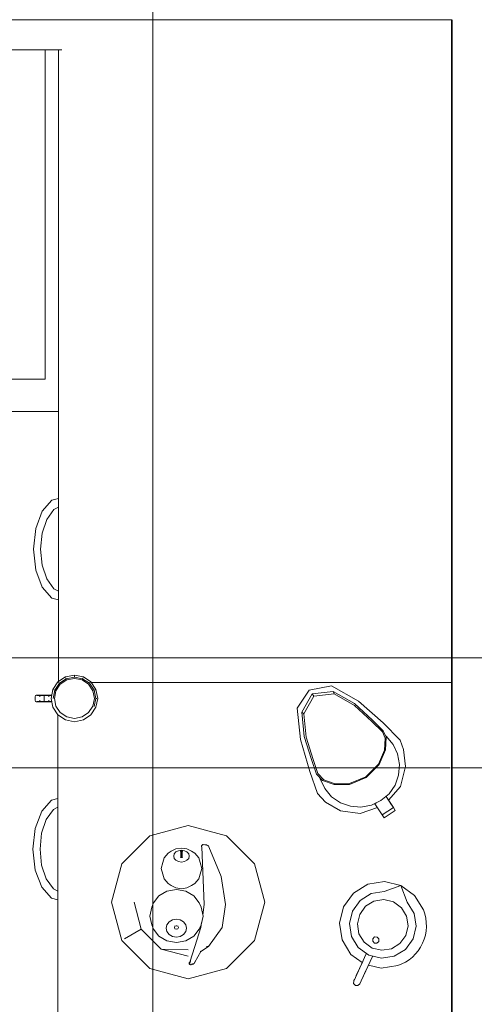
# Model space of a CAD drawing. Units: feet. Extents: x -297 to 770, y -228 to 625.
# Tile 12 of 14: x 716 to 734, y 194 to 233. Entities that reach past the tile are written whole.
import ezdxf

# ---------------------------------------------------------------- set-up
doc = ezdxf.new("R2010")
doc.units = ezdxf.units.FT
doc.header["$MEASUREMENT"] = 0
for name, color, linetype, lineweight in [('A-ANNO-DIMS', 2, 'Continuous', 18), ('A-EQPM', 8, 'Continuous', 13), ('A-FLOR-CASE', 8, 'Continuous', 18), ('A-FLOR-FIXT', 8, 'Continuous', 18), ('A-WALL', 7, 'Continuous', 35), ('windows', 30, 'Continuous', 18)]:
    doc.layers.add(name, color=color, linetype=linetype, lineweight=lineweight)
doc.styles.get("Standard").update_dxf_attribs({"font": 'arial.ttf'})
doc.dimstyles.get("Standard").update_dxf_attribs({"dimtxt": 3, "dimasz": 2, "dimexe": 0.18, "dimexo": 0.0625, "dimgap": 0.09, "dimtad": 1, "dimtoh": 1, "dimdec": 1, "dimzin": 0, "dimdsep": 46, "dimlunit": 3, "dimtxsty": 'Standard', "dimcen": 0, "dimclre": 256, "dimadec": 0, "dimazin": 0, "dimtfac": 1, "dimtdec": 1, "dimtofl": 0, "dimtmove": 0, "dimatfit": 3, "dimfxl": 1, "dimtolj": 1, "dimtzin": 0, "dimlwe": -1, "dimarcsym": 0})

# ---------------------------------------------------------------- blocks, each defined once
blk = doc.blocks.new('WIN-5FT')
blk.add_lwpolyline([(60, 0), (60, 9), (0, 9), (0, 0)], close=True)
blk = doc.blocks.new('*D54')
at = {"layer": 'A-ANNO-DIMS', "transparency": 16777216}
for p, q in [((733.096, 233.463), (354.525, 233.463)), ((733.093, 203.463), (354.525, 203.463))]:
    blk.add_line(p, q, dxfattribs=at)
at = {"layer": 'A-ANNO-DIMS', "color": 0, "lineweight": -2, "transparency": 16777216}
blk.add_line((354.705, 205.463), (354.705, 231.463), dxfattribs=at)
at = {"layer": 'A-ANNO-DIMS', "color": 0, "transparency": 16777216}
for points in [[(354.372, 231.463), (355.039, 231.463), (354.705, 233.463)], [(354.372, 205.463), (355.039, 205.463), (354.705, 203.463)]]:
    blk.add_solid(points, dxfattribs=at)
at = {"layer": 'Defpoints', "color": 0, "transparency": 16777216}
for p in [(354.705, 233.463), (733.158, 233.463), (733.155, 203.463)]:
    blk.add_point(p, dxfattribs=at)
at = {"layer": 'A-ANNO-DIMS', "color": 0, "transparency": 16777216, "insert": (353.083, 218.463), "char_height": 3, "attachment_point": 5, "rotation": 90}
blk.add_mtext('\\A1;30', dxfattribs=at)
blk = doc.blocks.new('*D68')
at = {"layer": 'A-ANNO-DIMS', "transparency": 16777216}
for p, q in [((685.155, 306.9), (685.155, -227.667)), ((721.155, 306.9), (721.155, -227.667))]:
    blk.add_line(p, q, dxfattribs=at)
at = {"layer": 'A-ANNO-DIMS', "color": 0, "lineweight": -2, "transparency": 16777216}
blk.add_line((687.155, -227.487), (719.155, -227.487), dxfattribs=at)
at = {"layer": 'A-ANNO-DIMS', "color": 0, "transparency": 16777216}
for points in [[(687.155, -227.154), (687.155, -227.821), (685.155, -227.487)], [(719.155, -227.154), (719.155, -227.821), (721.155, -227.487)]]:
    blk.add_solid(points, dxfattribs=at)
at = {"layer": 'Defpoints', "color": 0, "transparency": 16777216}
for p in [(685.155, 306.963), (721.155, 306.963), (721.155, -227.487)]:
    blk.add_point(p, dxfattribs=at)
at = {"layer": 'A-ANNO-DIMS', "color": 0, "transparency": 16777216, "insert": (703.155, -225.865), "char_height": 3, "attachment_point": 5}
blk.add_mtext('\\A1;36', dxfattribs=at)
blk = doc.blocks.new('*D75')
at = {"layer": 'A-ANNO-DIMS', "transparency": 16777216}
for p, q in [((471.753, 264.961), (769.785, 264.961)), ((471.753, 207.869), (769.785, 207.869))]:
    blk.add_line(p, q, dxfattribs=at)
at = {"layer": 'A-ANNO-DIMS', "color": 0, "lineweight": -2, "transparency": 16777216}
blk.add_line((769.605, 209.869), (769.605, 262.961), dxfattribs=at)
at = {"layer": 'A-ANNO-DIMS', "color": 0, "transparency": 16777216}
for points in [[(769.272, 262.961), (769.939, 262.961), (769.605, 264.961)], [(769.272, 209.869), (769.939, 209.869), (769.605, 207.869)]]:
    blk.add_solid(points, dxfattribs=at)
at = {"layer": 'Defpoints', "color": 0, "transparency": 16777216}
for p in [(471.691, 264.961), (769.605, 264.961), (471.691, 207.869)]:
    blk.add_point(p, dxfattribs=at)
at = {"layer": 'A-ANNO-DIMS', "color": 0, "transparency": 16777216, "insert": (767.984, 236.415), "char_height": 3, "attachment_point": 5, "rotation": 90}
blk.add_mtext('\\A1;57.09', dxfattribs=at)

msp = doc.modelspace()

# ---------------------------------------------------------------- linework, layer by layer
at = {"layer": 'A-EQPM'}
for p, q in [((726.947, 205.85), (727.438, 206.573)), ((727.438, 206.573), (728.324, 206.741)), ((728.324, 206.741), (729.408, 206.128)), ((727.141, 205.692), (727.547, 206.419)), ((727.614, 206.325), (727.222, 205.624)), ((727.547, 206.419), (728.394, 206.518)), ((727.547, 206.419), (727.614, 206.325)), ((728.43, 206.421), (727.614, 206.325)), ((728.394, 206.518), (729.252, 206.034)), ((728.394, 206.518), (728.43, 206.421)), ((729.257, 205.954), (728.43, 206.421)), ((727.084, 204.589), (726.947, 205.85)), ((729.252, 206.034), (729.972, 205.372)), ((729.951, 205.315), (729.257, 205.954)), ((730.4, 205.266), (729.408, 206.128)), ((727.235, 204.717), (727.141, 205.692)), ((727.141, 205.692), (727.222, 205.624)), ((727.222, 205.624), (727.313, 204.684)), ((729.972, 205.372), (730.407, 204.939)), ((730.371, 204.898), (729.951, 205.315)), ((731.087, 204.567), (730.4, 205.266)), ((727.084, 204.589), (727.462, 203.311)), ((727.53, 203.789), (727.235, 204.717)), ((727.313, 204.684), (727.597, 203.789)), ((730.484, 204.651), (730.371, 204.898)), ((730.407, 204.939), (730.525, 204.683)), ((730.451, 204.168), (730.484, 204.651)), ((730.525, 204.683), (730.49, 204.181)), ((730.522, 204.722), (730.5, 204.737)), ((730.798, 204.397), (730.522, 204.722)), ((731.087, 204.567), (731.221, 204.198)), ((730.211, 203.598), (730.451, 204.168)), ((730.49, 204.181), (730.241, 203.59)), ((730.981, 204.013), (730.798, 204.397)), ((731.221, 204.198), (731.296, 203.514)), ((727.725, 203.203), (727.53, 203.789)), ((727.597, 203.789), (727.785, 203.225)), ((731.058, 203.593), (730.981, 204.013)), ((729.705, 203.091), (730.211, 203.598)), ((730.241, 203.59), (729.717, 203.065)), ((731.023, 203.169), (731.058, 203.593)), ((731.296, 203.514), (731.101, 202.703)), ((727.462, 203.311), (727.772, 202.422)), ((727.97, 202.951), (727.725, 203.203)), ((727.785, 203.225), (728.021, 202.982)), ((727.866, 203.058), (727.875, 203.009)), ((727.875, 203.009), (728.058, 202.624)), ((728.021, 202.982), (728.471, 202.821)), ((729.717, 203.065), (729.045, 202.791)), ((729.058, 202.828), (729.705, 203.091)), ((730.881, 202.767), (731.023, 203.169)), ((728.437, 202.784), (727.97, 202.951)), ((728.058, 202.624), (728.334, 202.299)), ((729.045, 202.791), (728.437, 202.784)), ((728.471, 202.821), (729.058, 202.828)), ((731.101, 202.703), (730.616, 202.166)), ((730.639, 202.417), (730.881, 202.767)), ((727.772, 202.422), (728.092, 202.074)), ((728.334, 202.299), (728.685, 202.058)), ((730.314, 202.14), (730.639, 202.417)), ((730.524, 202.309), (730.476, 202.278)), ((730.742, 201.972), (730.524, 202.309)), ((730.524, 202.309), (730.603, 202.186)), ((730.814, 201.86), (730.524, 202.309)), ((728.092, 202.074), (728.686, 201.733)), ((728.685, 202.058), (729.086, 201.915)), ((729.086, 201.915), (729.511, 201.881)), ((729.486, 201.62), (730.174, 201.865)), ((729.511, 201.881), (729.93, 201.958)), ((729.93, 201.958), (730.314, 202.14)), ((730.075, 202.018), (730.123, 202.049)), ((730.365, 201.569), (730.075, 202.018)), ((730.365, 201.569), (730.814, 201.86)), ((730.814, 201.86), (730.742, 201.972)), ((730.788, 201.901), (730.814, 201.86)), ((730.814, 201.86), (730.887, 201.748)), ((728.686, 201.733), (729.486, 201.62)), ((730.438, 201.457), (730.365, 201.569)), ((730.887, 201.748), (730.438, 201.457)), ((722.574, 201.143), (721.036, 200.731)), ((722.574, 201.142), (721.037, 200.73)), ((724.111, 200.731), (722.574, 201.143)), ((724.111, 200.73), (722.574, 201.142)), ((721.036, 200.731), (719.911, 199.606)), ((721.037, 200.73), (719.912, 199.605)), ((725.237, 199.606), (724.111, 200.731)), ((725.236, 199.605), (724.111, 200.73)), ((722.308, 200.236), (722.087, 200.203)), ((722.529, 200.203), (722.308, 200.236)), ((723.111, 200.334), (723.12, 200.342)), ((723.114, 200.286), (723.111, 200.334)), ((723.111, 200.334), (723.113, 200.286)), ((723.113, 200.286), (723.114, 200.286)), ((723.114, 200.286), (723.114, 200.286)), ((723.119, 200.348), (723.134, 200.362)), ((723.146, 200.357), (723.119, 200.348)), ((723.119, 200.342), (723.119, 200.348)), ((723.224, 197.969), (723.122, 200.286)), ((723.134, 200.362), (723.139, 200.364)), ((723.134, 200.362), (723.151, 200.362)), ((723.142, 200.367), (723.139, 200.364)), ((723.139, 200.364), (723.142, 200.367)), ((723.153, 200.371), (723.142, 200.367)), ((723.171, 200.376), (723.153, 200.371)), ((723.155, 200.371), (723.171, 200.376)), ((723.16, 200.371), (723.171, 200.376)), ((723.171, 200.376), (723.168, 200.371)), ((723.171, 200.376), (723.259, 200.371)), ((723.206, 200.371), (723.171, 200.376)), ((723.171, 200.376), (723.22, 200.371)), ((723.171, 200.376), (723.179, 200.371)), ((723.259, 200.371), (723.292, 200.364)), ((723.286, 200.362), (723.27, 200.364)), ((723.312, 200.362), (723.292, 200.364)), ((723.325, 200.357), (723.312, 200.362)), ((723.344, 200.353), (723.325, 200.357)), ((723.344, 200.353), (723.372, 200.338)), ((723.383, 200.334), (723.37, 200.339)), ((723.38, 200.332), (723.383, 200.334)), ((723.383, 200.334), (723.384, 200.332)), ((723.384, 200.332), (723.39, 200.329)), ((723.39, 200.329), (723.408, 200.286)), ((723.408, 200.286), (723.395, 200.286)), ((723.898, 199.095), (723.403, 200.286)), ((721.611, 199.844), (721.554, 199.657)), ((721.775, 200.029), (721.611, 199.844)), ((721.9, 200.108), (721.775, 200.029)), ((722.087, 200.203), (721.9, 200.108)), ((722.019, 200.006), (721.996, 199.916)), ((721.996, 199.916), (722.019, 199.826)), ((722.087, 200.083), (722.019, 200.006)), ((722.019, 199.826), (722.087, 199.749)), ((722.188, 200.134), (722.087, 200.083)), ((722.308, 200.152), (722.188, 200.134)), ((722.267, 200.117), (722.279, 200.125)), ((722.279, 200.108), (722.267, 200.117)), ((722.267, 200.117), (722.279, 200.059)), ((722.279, 199.906), (722.269, 199.87)), ((722.279, 200.125), (722.308, 200.129)), ((722.287, 200.051), (722.279, 200.108)), ((722.279, 200.108), (722.308, 200.105)), ((722.279, 200.059), (722.285, 200.004)), ((722.285, 199.953), (722.279, 199.906)), ((722.28, 199.849), (722.287, 199.892)), ((722.285, 200.004), (722.285, 199.953)), ((722.292, 199.996), (722.287, 200.051)), ((722.287, 199.892), (722.292, 199.943)), ((722.292, 199.943), (722.292, 199.996)), ((722.428, 200.134), (722.308, 200.152)), ((722.308, 200.129), (722.337, 200.125)), ((722.308, 200.105), (722.337, 200.108)), ((722.308, 200.105), (722.308, 199.841)), ((722.329, 200.051), (722.324, 199.996)), ((722.324, 199.996), (722.324, 199.943)), ((722.324, 199.943), (722.329, 199.892)), ((722.337, 200.108), (722.329, 200.051)), ((722.329, 199.892), (722.336, 199.849)), ((722.337, 200.059), (722.331, 200.004)), ((722.331, 200.004), (722.331, 199.953)), ((722.331, 199.953), (722.337, 199.906)), ((722.337, 200.125), (722.349, 200.117)), ((722.337, 200.108), (722.349, 200.117)), ((722.349, 200.117), (722.337, 200.059)), ((722.337, 199.906), (722.347, 199.87)), ((722.529, 200.083), (722.428, 200.134)), ((722.716, 200.108), (722.529, 200.203)), ((722.597, 200.006), (722.529, 200.083)), ((722.529, 199.749), (722.597, 199.826)), ((722.62, 199.916), (722.597, 200.006)), ((722.597, 199.826), (722.62, 199.916)), ((722.841, 200.029), (722.716, 200.108)), ((723.005, 199.844), (722.841, 200.029)), ((723.062, 199.657), (723.005, 199.844)), ((719.911, 199.606), (719.499, 198.068)), ((719.912, 199.605), (719.5, 198.068)), ((721.554, 199.657), (721.492, 199.421)), ((722.087, 199.749), (722.188, 199.698)), ((722.188, 199.698), (722.308, 199.68)), ((722.308, 199.68), (722.428, 199.698)), ((722.428, 199.698), (722.529, 199.749)), ((723.124, 199.421), (723.062, 199.657)), ((725.648, 198.068), (725.236, 199.605)), ((725.649, 198.068), (725.237, 199.606)), ((721.492, 199.421), (721.554, 199.186)), ((721.554, 199.186), (721.611, 198.999)), ((723.005, 198.999), (723.062, 199.186)), ((723.062, 199.186), (723.124, 199.421)), ((724.078, 197.969), (723.898, 199.095)), ((721.611, 198.999), (721.775, 198.814)), ((721.775, 198.814), (721.9, 198.735)), ((721.9, 198.735), (722.087, 198.64)), ((722.087, 198.64), (722.308, 198.607)), ((722.308, 198.607), (722.529, 198.64)), ((722.529, 198.64), (722.716, 198.735)), ((722.716, 198.735), (722.841, 198.814)), ((722.841, 198.814), (723.005, 198.999)), ((729.784, 198.786), (729.206, 198.431)), ((730.454, 198.893), (729.784, 198.786)), ((731.113, 198.735), (730.438, 198.492)), ((731.113, 198.735), (730.454, 198.893)), ((731.662, 198.337), (731.113, 198.735)), ((731.368, 198.064), (731.113, 198.735)), ((721.405, 198.321), (721.191, 198.042)), ((721.725, 198.508), (721.405, 198.321)), ((722.104, 198.573), (721.725, 198.508)), ((722.482, 198.508), (722.104, 198.573)), ((722.802, 198.321), (722.482, 198.508)), ((723.017, 198.042), (722.802, 198.321)), ((729.206, 198.431), (728.808, 197.882)), ((729.923, 198.41), (729.478, 198.137)), ((730.438, 198.492), (729.923, 198.41)), ((732.017, 197.758), (731.662, 198.337)), ((719.499, 198.068), (719.911, 196.53)), ((719.5, 198.068), (719.912, 196.531)), ((720.695, 196.983), (720.404, 198.068)), ((721.115, 197.868), (721.034, 197.511)), ((721.191, 198.042), (721.115, 197.868)), ((723.092, 197.868), (723.017, 198.042)), ((723.173, 197.511), (723.092, 197.868)), ((723.162, 197.562), (723.224, 197.969)), ((723.946, 197.059), (724.078, 197.969)), ((725.236, 196.531), (725.648, 198.068)), ((725.237, 196.53), (725.649, 198.068)), ((728.808, 197.882), (728.65, 197.222)), ((729.478, 198.137), (729.172, 197.714)), ((729.695, 197.903), (729.462, 197.581)), ((730.033, 198.111), (729.695, 197.903)), ((730.426, 198.173), (730.033, 198.111)), ((730.812, 198.081), (730.426, 198.173)), ((731.134, 197.847), (730.812, 198.081)), ((731.342, 197.509), (731.134, 197.847)), ((731.641, 197.619), (731.368, 198.064)), ((721.034, 197.511), (721.115, 197.155)), ((723.092, 197.155), (723.173, 197.511)), ((729.172, 197.714), (729.051, 197.207)), ((729.462, 197.581), (729.369, 197.195)), ((731.404, 197.116), (731.342, 197.509)), ((731.723, 197.104), (731.641, 197.619)), ((721.115, 197.155), (721.191, 196.981)), ((721.725, 197.161), (721.694, 197.025)), ((721.814, 197.277), (721.725, 197.161)), ((721.947, 197.354), (721.814, 197.277)), ((722.104, 197.381), (721.947, 197.354)), ((722.023, 197.051), (722.047, 197.1)), ((722.023, 197.051), (722.023, 197.067)), ((722.047, 197.1), (722.104, 197.121)), ((722.047, 197.1), (722.047, 197.116)), ((722.26, 197.354), (722.104, 197.381)), ((722.104, 197.121), (722.104, 197.137)), ((722.104, 197.121), (722.16, 197.1)), ((722.16, 197.1), (722.16, 197.116)), ((722.16, 197.1), (722.184, 197.051)), ((722.184, 197.051), (722.184, 197.067)), ((722.393, 197.277), (722.26, 197.354)), ((722.482, 197.161), (722.393, 197.277)), ((722.513, 197.025), (722.482, 197.161)), ((722.85, 196.286), (723.084, 197.059)), ((723.017, 196.981), (723.092, 197.155)), ((723.084, 197.059), (723.114, 197.253)), ((723.388, 196.286), (723.946, 197.059)), ((728.65, 197.222), (728.756, 196.553)), ((729.051, 197.207), (729.133, 196.692)), ((729.369, 197.195), (729.432, 196.802)), ((731.312, 196.73), (731.404, 197.116)), ((731.601, 196.597), (731.723, 197.104)), ((720.027, 196.597), (720.695, 196.983)), ((720.695, 196.983), (721.489, 196.188)), ((721.191, 196.981), (721.405, 196.702)), ((721.405, 196.702), (721.725, 196.515)), ((721.694, 197.025), (721.725, 196.889)), ((721.725, 196.889), (721.814, 196.773)), ((721.814, 196.773), (721.947, 196.696)), ((721.947, 196.696), (722.104, 196.669)), ((722.047, 197.001), (722.023, 197.051)), ((722.104, 196.981), (722.047, 197.001)), ((722.16, 197.001), (722.104, 196.981)), ((722.104, 196.669), (722.26, 196.696)), ((722.184, 197.051), (722.16, 197.001)), ((722.26, 196.696), (722.393, 196.773)), ((722.393, 196.773), (722.482, 196.889)), ((722.482, 196.889), (722.513, 197.025)), ((722.482, 196.515), (722.802, 196.702)), ((722.802, 196.702), (723.017, 196.981)), ((729.133, 196.692), (729.406, 196.247)), ((729.432, 196.802), (729.639, 196.464)), ((729.986, 196.604), (730.061, 196.674)), ((730.061, 196.674), (730.163, 196.67)), ((730.163, 196.67), (730.233, 196.595)), ((731.078, 196.408), (731.312, 196.73)), ((719.911, 196.53), (721.036, 195.404)), ((719.912, 196.531), (721.037, 195.405)), ((721.725, 196.515), (722.104, 196.45)), ((722.104, 196.45), (722.482, 196.515)), ((722.637, 195.66), (722.85, 196.286)), ((723.086, 196.091), (723.388, 196.286)), ((723.388, 196.286), (723.309, 196.286)), ((724.111, 195.405), (725.236, 196.531)), ((724.111, 195.404), (725.237, 196.53)), ((728.756, 196.553), (729.111, 195.975)), ((729.639, 196.464), (729.961, 196.23)), ((729.982, 196.502), (729.986, 196.604)), ((730.051, 196.427), (729.982, 196.502)), ((730.154, 196.423), (730.051, 196.427)), ((730.229, 196.492), (730.154, 196.423)), ((730.233, 196.595), (730.229, 196.492)), ((730.74, 196.2), (731.078, 196.408)), ((731.295, 196.174), (731.601, 196.597)), ((721.489, 196.188), (722.574, 196.161)), ((721.489, 196.188), (722.574, 195.898)), ((722.848, 195.66), (723.086, 196.091)), ((723.059, 196.1), (723.086, 196.091)), ((729.111, 195.975), (729.563, 195.647)), ((729.221, 194.905), (729.725, 196.001)), ((729.406, 196.247), (729.828, 195.941)), ((729.521, 194.917), (729.971, 195.894)), ((729.828, 195.941), (730.335, 195.819)), ((729.961, 196.23), (730.347, 196.138)), ((730.335, 195.819), (730.85, 195.901)), ((730.347, 196.138), (730.74, 196.2)), ((730.85, 195.901), (731.295, 196.174)), ((722.615, 195.611), (722.622, 195.636)), ((722.62, 195.611), (722.615, 195.611)), ((722.615, 195.611), (722.619, 195.587)), ((722.619, 195.587), (722.62, 195.619)), ((722.619, 195.587), (722.628, 195.578)), ((722.63, 195.587), (722.619, 195.587)), ((722.62, 195.619), (722.637, 195.66)), ((722.62, 195.619), (722.629, 195.611)), ((722.637, 195.66), (722.622, 195.636)), ((722.622, 195.636), (722.628, 195.639)), ((722.622, 195.636), (722.627, 195.636)), ((722.628, 195.578), (722.639, 195.57)), ((722.629, 195.611), (722.645, 195.652)), ((722.643, 195.604), (722.629, 195.611)), ((722.629, 195.611), (722.642, 195.587)), ((722.629, 195.611), (722.63, 195.587)), ((722.63, 195.587), (722.634, 195.578)), ((722.642, 195.587), (722.63, 195.587)), ((722.634, 195.578), (722.642, 195.587)), ((722.635, 195.652), (722.651, 195.66)), ((722.635, 195.652), (722.64, 195.66)), ((722.645, 195.652), (722.635, 195.652)), ((722.64, 195.66), (722.637, 195.66)), ((722.639, 195.57), (722.69, 195.562)), ((722.651, 195.66), (722.64, 195.66)), ((722.645, 195.611), (722.64, 195.611)), ((722.69, 195.562), (722.64, 195.57)), ((722.642, 195.587), (722.645, 195.611)), ((722.645, 195.57), (722.69, 195.562)), ((722.65, 195.699), (722.682, 195.699)), ((722.668, 195.66), (722.651, 195.66)), ((722.69, 195.562), (722.651, 195.57)), ((722.69, 195.562), (722.67, 195.57)), ((722.681, 195.57), (722.69, 195.562)), ((722.723, 195.57), (722.69, 195.562)), ((722.69, 195.562), (722.717, 195.57)), ((722.702, 195.57), (722.69, 195.562)), ((722.69, 195.562), (722.721, 195.57)), ((722.69, 195.562), (722.71, 195.57)), ((722.69, 195.562), (722.692, 195.57)), ((722.721, 195.57), (722.741, 195.578)), ((722.739, 195.577), (722.723, 195.57)), ((722.727, 195.595), (722.748, 195.595)), ((722.73, 195.579), (722.75, 195.587)), ((722.739, 195.577), (722.772, 195.587)), ((722.748, 195.595), (722.754, 195.596)), ((722.772, 195.587), (722.823, 195.611)), ((722.819, 195.611), (722.786, 195.603)), ((722.819, 195.611), (722.792, 195.611)), ((722.814, 195.608), (722.819, 195.611)), ((722.819, 195.611), (722.848, 195.66)), ((722.823, 195.611), (722.819, 195.611)), ((722.823, 195.611), (722.821, 195.614)), ((722.848, 195.66), (722.823, 195.611)), ((722.84, 195.652), (722.83, 195.652)), ((722.833, 195.66), (722.848, 195.66)), ((722.833, 195.66), (722.84, 195.652)), ((722.848, 195.66), (722.84, 195.652)), ((729.322, 195.125), (729.584, 195.692)), ((729.808, 195.541), (730.32, 195.419)), ((730.32, 195.419), (730.989, 195.525)), ((721.036, 195.404), (722.574, 194.992)), ((721.037, 195.405), (722.574, 194.993)), ((722.574, 194.993), (724.111, 195.405)), ((722.574, 194.992), (724.111, 195.404)), ((729.599, 195.086), (729.708, 195.323)), ((729.217, 194.803), (729.221, 194.905)), ((729.217, 194.803), (729.287, 194.728)), ((729.221, 194.905), (729.229, 194.922)), ((729.229, 194.922), (729.248, 194.963)), ((729.287, 194.728), (729.389, 194.724)), ((729.389, 194.724), (729.464, 194.793)), ((729.464, 194.793), (729.521, 194.917)), ((729.482, 194.832), (729.572, 195.027))]:
    msp.add_line(p, q, dxfattribs=at)
msp.add_arc((730.453, 197.125), 1.687, 288.5386, 22.0579, dxfattribs=at)
at = {"layer": 'A-FLOR-CASE'}
for p, q in [((680.083, 233.463), (733.158, 233.463)), ((733.155, 113.516), (733.155, 233.463)), ((717.37, 217.912), (717.37, 232.254)), ((696.125, 217.748), (717.37, 217.748)), ((717.37, 206.918), (717.37, 217.912)), ((717.107, 214.187), (716.721, 213.752)), ((717.107, 214.187), (717.37, 214.254)), ((716.721, 213.752), (716.458, 213.06)), ((717.19, 213.816), (716.901, 213.418)), ((717.37, 213.908), (717.19, 213.816)), ((716.901, 213.418), (716.715, 212.863)), ((716.458, 213.06), (716.365, 212.225)), ((716.715, 212.863), (716.65, 212.225)), ((716.365, 212.225), (716.458, 211.391)), ((716.65, 212.225), (716.715, 211.588)), ((716.458, 211.391), (716.721, 210.699)), ((716.715, 211.588), (716.901, 211.032)), ((716.901, 211.032), (717.19, 210.634)), ((716.721, 210.699), (717.107, 210.264)), ((717.19, 210.634), (717.37, 210.543)), ((717.107, 210.264), (717.37, 210.196)), ((717.35, 206.905), (717.654, 207.108)), ((717.407, 206.848), (717.685, 207.033)), ((717.705, 206.984), (717.445, 206.811)), ((717.654, 207.108), (718.012, 207.179)), ((717.685, 207.033), (717.668, 207.073)), ((717.685, 207.033), (718.012, 207.099)), ((718.012, 207.046), (717.705, 206.984)), ((718.012, 207.179), (718.37, 207.108)), ((718.012, 207.099), (718.012, 207.141)), ((718.012, 207.099), (718.339, 207.033)), ((718.319, 206.984), (718.012, 207.046)), ((718.579, 206.811), (718.319, 206.984)), ((718.339, 207.033), (718.355, 207.073)), ((718.339, 207.033), (718.616, 206.848)), ((718.37, 207.108), (718.674, 206.905)), ((717.076, 206.243), (717.147, 206.601)), ((717.147, 206.601), (717.35, 206.905)), ((717.157, 206.243), (717.222, 206.571)), ((717.222, 206.571), (717.182, 206.587)), ((717.271, 206.55), (717.21, 206.243)), ((717.222, 206.571), (717.407, 206.848)), ((717.445, 206.811), (717.271, 206.55)), ((717.407, 206.848), (717.377, 206.878)), ((718.753, 206.55), (718.579, 206.811)), ((718.616, 206.848), (718.647, 206.878)), ((718.616, 206.848), (718.802, 206.571)), ((718.674, 206.905), (718.876, 206.601)), ((718.69, 206.88), (733.155, 206.88)), ((718.814, 206.243), (718.753, 206.55)), ((718.802, 206.571), (718.841, 206.587)), ((718.867, 206.243), (718.802, 206.571)), ((718.876, 206.601), (718.948, 206.243)), ((716.441, 206.306), (716.437, 206.239)), ((716.437, 206.239), (716.441, 206.172)), ((716.453, 206.355), (716.441, 206.306)), ((716.441, 206.172), (716.453, 206.123)), ((716.47, 206.373), (716.453, 206.355)), ((716.515, 206.373), (716.47, 206.373)), ((716.5, 206.355), (716.629, 206.355)), ((716.637, 206.373), (716.515, 206.373)), ((716.629, 206.355), (716.623, 206.306)), ((716.623, 206.172), (716.629, 206.123)), ((716.629, 206.355), (716.637, 206.373)), ((716.804, 206.355), (716.629, 206.355)), ((716.637, 206.373), (716.804, 206.373)), ((716.971, 206.373), (716.804, 206.373)), ((716.804, 206.373), (716.804, 206.355)), ((716.804, 206.355), (716.98, 206.355)), ((716.804, 206.123), (716.804, 206.355)), ((716.971, 206.373), (717.102, 206.373)), ((716.98, 206.355), (716.971, 206.373)), ((717.098, 206.355), (716.98, 206.355)), ((716.98, 206.355), (716.986, 206.306)), ((716.98, 206.123), (716.986, 206.172)), ((717.147, 205.885), (717.076, 206.243)), ((717.076, 206.243), (717.077, 206.239)), ((717.077, 206.239), (717.082, 206.212)), ((717.094, 206.333), (717.098, 206.355)), ((717.098, 206.355), (717.099, 206.361)), ((717.21, 206.243), (717.271, 205.936)), ((718.753, 205.936), (718.814, 206.243)), ((718.802, 205.916), (718.867, 206.243)), ((718.867, 206.243), (718.91, 206.243)), ((718.948, 206.243), (718.876, 205.885)), ((716.453, 206.123), (716.47, 206.105)), ((716.47, 206.105), (716.637, 206.105)), ((716.629, 206.123), (716.5, 206.123)), ((716.629, 206.123), (716.804, 206.123)), ((716.637, 206.105), (716.629, 206.123)), ((716.804, 206.105), (716.637, 206.105)), ((716.98, 206.123), (716.804, 206.123)), ((716.804, 206.123), (716.804, 206.105)), ((716.804, 206.105), (716.971, 206.105)), ((716.971, 206.105), (716.98, 206.123)), ((716.971, 206.105), (717.103, 206.105)), ((717.1, 206.123), (716.98, 206.123)), ((717.35, 205.581), (717.147, 205.885)), ((717.271, 205.936), (717.445, 205.676)), ((718.579, 205.676), (718.753, 205.936)), ((718.876, 205.885), (718.674, 205.581)), ((717.654, 205.379), (717.35, 205.581)), ((717.351, 180.136), (717.351, 205.581)), ((717.445, 205.676), (717.705, 205.502)), ((718.012, 205.307), (717.654, 205.379)), ((717.705, 205.502), (718.012, 205.441)), ((718.012, 205.441), (718.319, 205.502)), ((718.37, 205.379), (718.012, 205.307)), ((718.319, 205.502), (718.579, 205.676)), ((718.674, 205.581), (718.37, 205.379)), ((717.088, 202.156), (717.351, 202.223)), ((717.088, 202.156), (716.703, 201.72)), ((717.351, 201.877), (717.171, 201.785)), ((716.703, 201.72), (716.439, 201.028)), ((717.171, 201.785), (716.883, 201.387)), ((716.439, 201.028), (716.346, 200.193)), ((716.883, 201.387), (716.696, 200.831)), ((716.696, 200.831), (716.631, 200.193)), ((716.346, 200.193), (716.439, 199.358)), ((716.631, 200.193), (716.696, 199.555)), ((716.696, 199.555), (716.883, 199)), ((716.439, 199.358), (716.703, 198.666)), ((716.703, 198.666), (717.088, 198.23)), ((716.883, 199), (717.171, 198.601)), ((717.171, 198.601), (717.351, 198.509)), ((717.088, 198.23), (717.351, 198.163))]:
    msp.add_line(p, q, dxfattribs=at)
at = {"layer": 'A-FLOR-FIXT'}
for p, q in [((712.053, 232.254), (717.503, 232.254)), ((716.841, 219.047), (716.841, 232.254)), ((706.499, 219.047), (716.841, 219.047)), ((716.841, 219.047), (706.74, 219.047))]:
    msp.add_line(p, q, dxfattribs=at)
at = {"layer": 'A-WALL'}
msp.add_lwpolyline([(733.155, 113.463), (733.155, 233.463)], dxfattribs=at)

# ---------------------------------------------------------------- block references
at = {"layer": 'windows', "rotation": 90.00000000000003}
msp.add_blockref('WIN-5FT', (742.155, 143.463), dxfattribs=at)

# ---------------------------------------------------------------- dimensions: what is measured, and where the dimension line sits
at = {"layer": 'A-ANNO-DIMS'}
dim = msp.add_linear_dim(base=(721.155, -227.487), p1=(685.155, 306.963), p2=(721.155, 306.963), dimstyle='Standard', override={"dimdec": 0, "dimlfac": 1, "dimrnd": 0, "dimzin": 0, "dimdsep": 46, "dimlunit": 2}, dxfattribs=at)
dim.commit()
dim.dimension.update_dxf_attribs({"geometry": '*D68', "text_midpoint": (703.155, -225.865)})
for base, p1, p2, override, picture, middle in [((769.605, 264.961), (471.691, 207.869), (471.691, 264.961), {"dimdec": 2, "dimlfac": 1, "dimrnd": 0, "dimzin": 0, "dimdsep": 46, "dimlunit": 2}, '*D75', (767.984, 236.415)), ((354.705, 233.463), (733.155, 203.463), (733.158, 233.463), {"dimdec": 0, "dimlfac": 1, "dimrnd": 0, "dimzin": 0, "dimdsep": 46, "dimlunit": 2}, '*D54', (353.083, 218.463))]:
    dim = msp.add_linear_dim(base=base, p1=p1, p2=p2, angle=90, dimstyle='Standard', override=override, dxfattribs=at)
    dim.commit()
    dim.dimension.update_dxf_attribs({"geometry": picture, "text_midpoint": middle})

doc.saveas('drawing.dxf')
